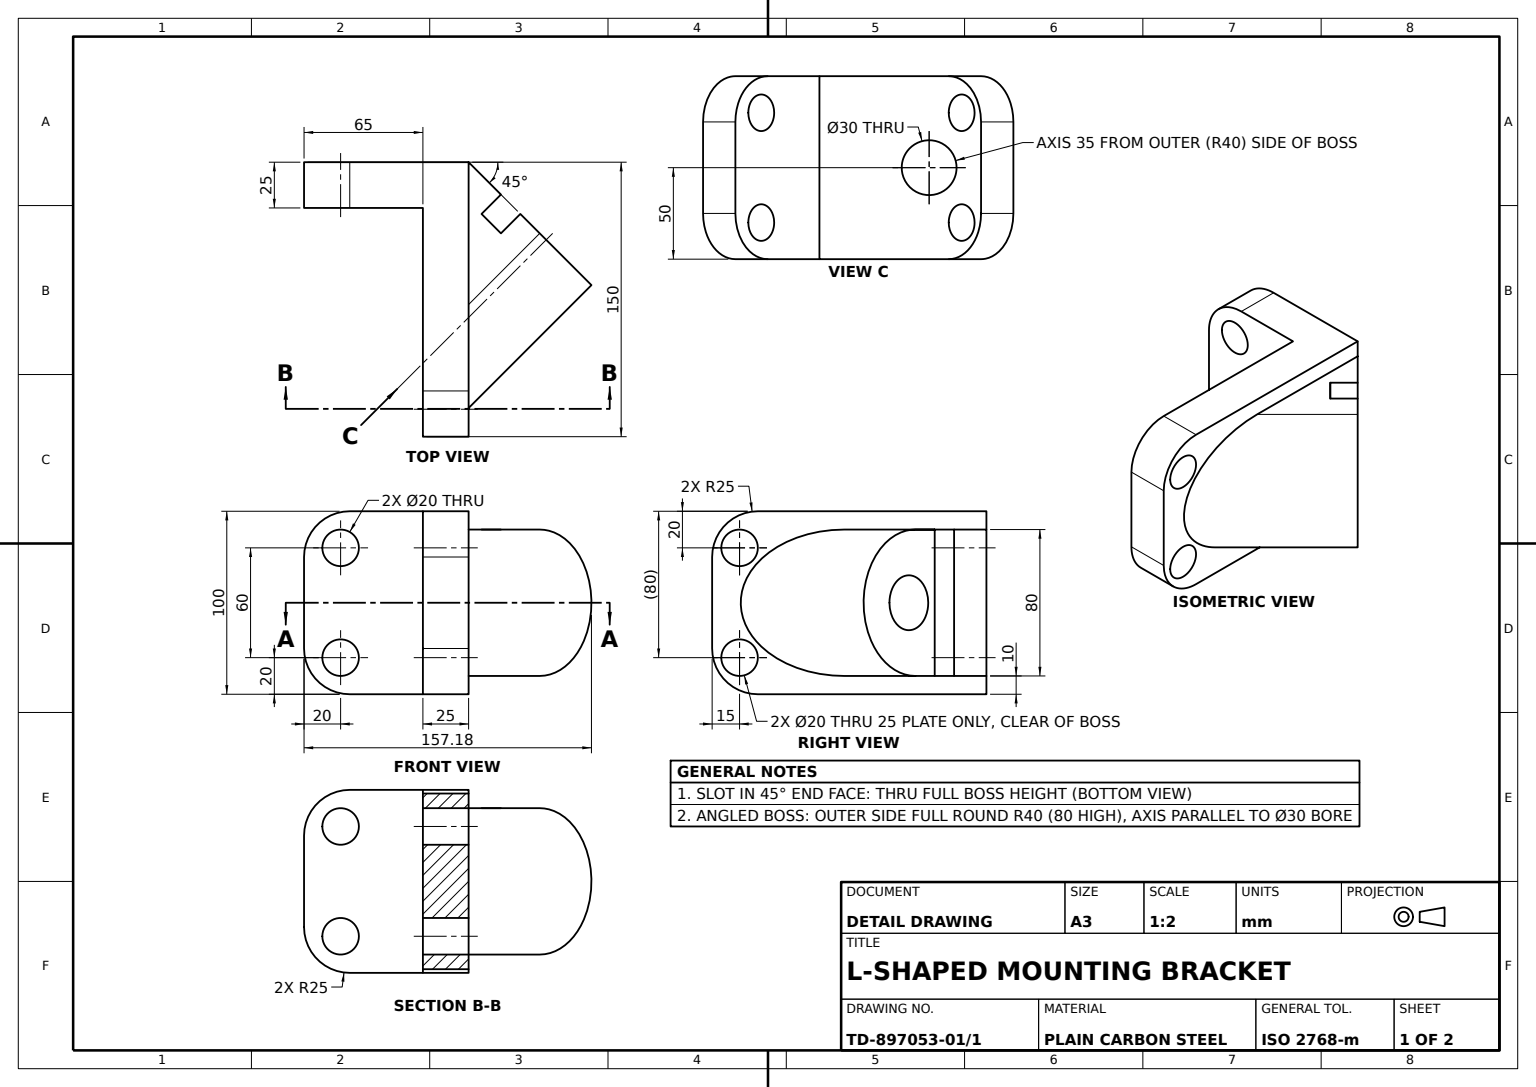
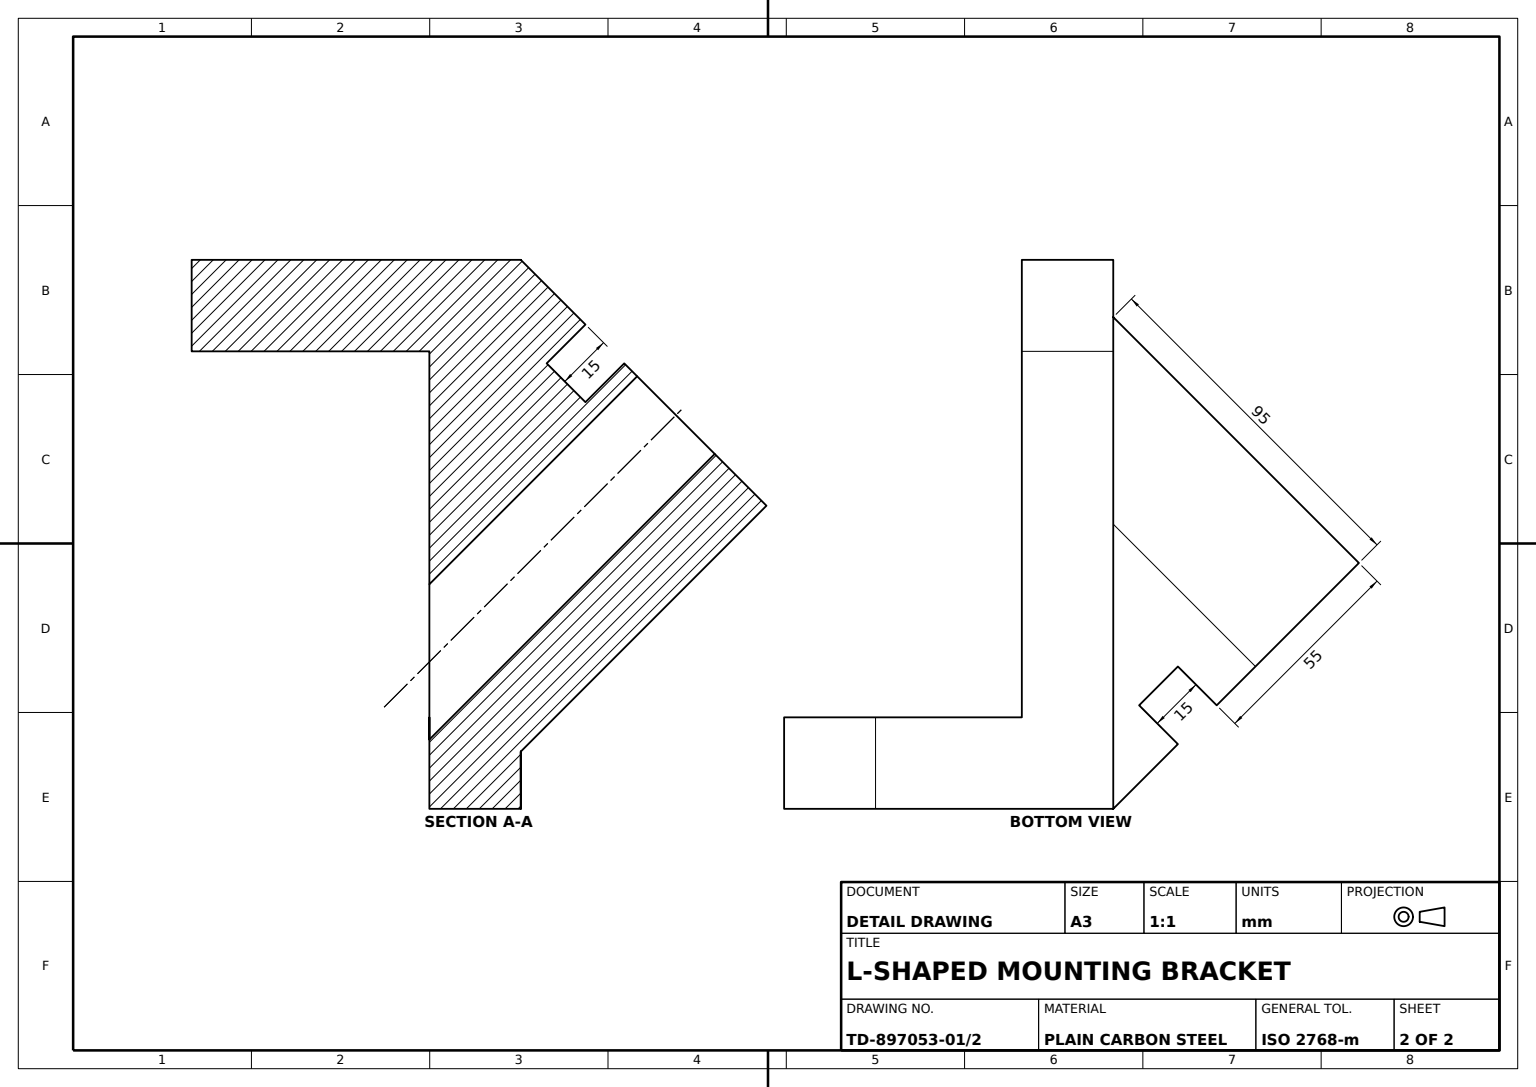
SolidWorks part; units mm, degrees
material "Plain Carbon Steel"
ref_plane "Front Plane" through (0, 0, 0) normal (0, 0, 1) x (1, 0, 0)
ref_plane "Top Plane" through (0, 0, 0) normal (0, 1, 0) x (1, 0, 0)
ref_plane "Right Plane" through (0, 0, 0) normal (1, 0, 0) x (0, 0, -1)
sketch "Base Plate Sketch" plane through (0, 0, 0) normal (0, 0, 1) x (1, 0, 0)
  line L1 (-75, -50) -> (75, -50)
  line L2 (-75, -50) -> (-75, 50)
  line L3 (-75, 50) -> (75, 50)
  line L4 (75, -50) -> (75, 50)
  line L5 (-75, -50) -> (75, 50) construction
  line L6 (-75, 50) -> (75, -50) construction
  point P0 (0, 0)
  dimension "D1" = 100
  dimension "D2" = 150
extrude "Base Plate 150x100x25" add sketch "Base Plate Sketch" along normal blind 25
sketch "Upright Plate Sketch" plane through (0, 0, 25) normal (0, 0, 1) x (1, 0, 0)
  line L0 (-75, -50) -> (75, -50) construction
  line L1 (-75, 50) -> (-50, 50)
  line L2 (-75, 50) -> (-75, -50)
  line L3 (-75, -50) -> (-50, -50)
  line L4 (-50, 50) -> (-50, -50)
  dimension "D1" = 25
extrude "Upright Plate" add sketch "Upright Plate Sketch" along normal blind 65
sketch "Boss Layout Sketch 45deg" plane through (0, 0, 0) normal (0, 1, 0) x (1, 0, 0)
  line L0 (75, 0) -> (-75, 0) construction
  line L1 (75, 0) -> (-75, 0)
  line L2 (-75, 0) -> (-7.8249, 67.1751)
  dimension "D1" = 45
  dimension "D2" = 95
ref_plane "Boss Reference Plane" through (0, 0, 0) normal (0, -1, 0) x (0.7071, 0, -0.7071)
ref_plane "Boss Sketch Plane" through (-37.5, 0, -37.5) normal (0.7071, 0, 0.7071) x (0.7071, 0, -0.7071)
sketch "Angled Boss Sketch" plane through (-37.5, 0, -37.5) normal (0.7071, 0, 0.7071) x (0.7071, 0, -0.7071)
  line L0 (-53.033, 0) -> (41.967, 0) construction
  line L1 (-53.033, -50) -> (-53.033, 50) construction
  line L2 (-53.033, 40) -> (1.967, 40)
  line L3 (-53.033, 40) -> (-53.033, -40)
  line L4 (-53.033, -40) -> (1.967, -40)
  line L6 (-53.033, -50) -> (35.3553, -50) construction
  line L7 (35.3553, 50) -> (-53.033, 50) construction
  arc A1 (1.967, -40) -> (1.967, 40) centre (1.967, 0) ccw
  dimension "D4" = 80
  dimension "D1" = 10
  dimension "D2" = 10
  dimension "D3" = 55
extrude "Angled Boss" add sketch "Angled Boss Sketch" along normal up to next
sketch "Boss Slot Sketch" plane through (0, 40, 0) normal (0, 1, 0) x (1, 0, 0)
  line L0 (-57.3223, 17.6777) -> (-46.7157, 7.0711)
  line L1 (-36.1091, 38.8909) -> (-75, 0) construction
  line L2 (-46.7157, 7.0711) -> (-36.1091, 17.6777)
  line L3 (-36.1091, 17.6777) -> (-46.7157, 28.2843)
  line L4 (-46.7157, 28.2843) -> (-57.3223, 17.6777)
  dimension "D1" = 25
  dimension "D2" = 15
  dimension "D3" = 15
  dimension "D4" = 38.8909
extrude "Boss Slot" cut sketch "Boss Slot Sketch" against normal up to next contours L3 L4 L0 L2
sketch "Boss Bore Sketch" plane through (-37.5, 0, -37.5) normal (-0.7071, 0, -0.7071) x (-0.7071, 0, 0.7071)
  line L0 (28.033, 0) -> (-6.967, 0) construction
  line L1 (28.033, -40) -> (28.033, 40) construction
  circle A0 centre (-6.967, 0) radius 15
  dimension "D2" = 30
  dimension "D1" = 35
extrude "Boss Bore" cut sketch "Boss Bore Sketch" against normal up to next
sketch "Base Plate Holes Sketch" plane through (0, 0, 0) normal (0, 0, -1) x (-1, 0, 0)
  line L0 (-105.8098, 0) -> (25.2569, 0) construction
  line L2 (-75, -50) -> (-75, 50) construction
  circle A0 centre (-60, 30) radius 10
  circle A1 centre (-60, -30) radius 10
  dimension "D1" = 20
  dimension "D2" = 20
  dimension "D3" = 60
  dimension "D4" = 15
extrude "Base Plate Holes" cut sketch "Base Plate Holes Sketch" against normal up to next
sketch "Upright Plate Holes Sketch" plane through (-75, 0, 0) normal (-1, 0, 0) x (0, 0, 1)
  line L0 (-20.317, 0) -> (135.1065, 0) construction
  line L1 (90, 50) -> (90, -50) construction
  line L2 (90, 50) -> (0, 50) construction
  circle A0 centre (70, 30) radius 10
  circle A1 centre (70, -30) radius 10
  dimension "D3" = 20
  dimension "D4" = 20
  dimension "D1" = 60
  dimension "D2" = 20
  dimension "D5" = 20
  dimension "D6" = 70
extrude "Upright Plate Holes" cut sketch "Upright Plate Holes Sketch" against normal up to next
fillet "Upright Corner Fillet R25 A" radius 25 1 edges at (-62.5, 50, 90)
fillet "Upright Corner Fillet R25 B" radius 25 1 edges at (-62.5, -50, 90)
fillet "Base Corner Fillet R25 A" radius 25 1 edges at (75, -50, 12.5)
fillet "Base Corner Fillet R25 B" radius 25 1 edges at (75, 50, 12.5)
equation "\"`5\"=5.89137"
